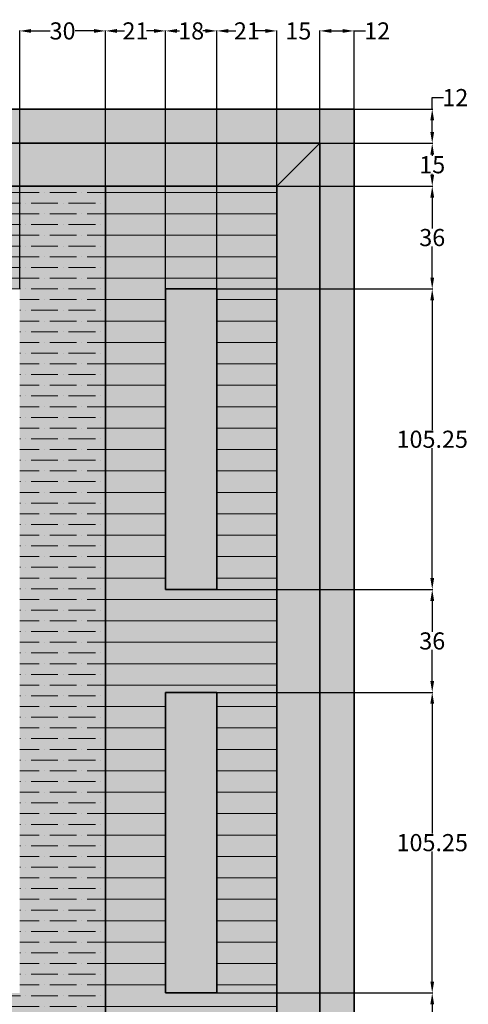
# Model space of a CAD drawing. Units: inches. Extents: x 184 to 649, y 215 to 818.
# Tile 9 of 9: x 492 to 649, y 473 to 818. Entities that reach past the tile are written whole.
import ezdxf

# ---------------------------------------------------------------- set-up
doc = ezdxf.new("R2010")
doc.units = ezdxf.units.IN
doc.header["$MEASUREMENT"] = 0
for name, color, linetype, lineweight in [('A-ANNO-DIMS', 2, 'Continuous', 18), ('A-ELEV', 7, 'Continuous', 35), ('A-ELEV-FILL', 9, 'Continuous', 13), ('A-ELEV-PATT', 8, 'Continuous', 13)]:
    doc.layers.add(name, color=color, linetype=linetype, lineweight=lineweight)
doc.styles.get("Standard").update_dxf_attribs({"font": 'arial.ttf'})
doc.dimstyles.get("Standard").update_dxf_attribs({"dimtxt": 6, "dimasz": 4, "dimexe": 0.18, "dimexo": 0.0625, "dimgap": 0.09, "dimtad": 0, "dimtih": 1, "dimtoh": 1, "dimdec": 0, "dimzin": 0, "dimdsep": 46, "dimlunit": 3, "dimtxsty": 'Standard', "dimcen": 0.09, "dimadec": 0, "dimazin": 0, "dimtfac": 1, "dimtdec": 0, "dimtofl": 0, "dimtmove": 0, "dimatfit": 3, "dimfxl": 1, "dimtolj": 1, "dimtzin": 0, "dimarcsym": 0})

# ---------------------------------------------------------------- blocks, each defined once
blk = doc.blocks.new('*D23')
at = {"layer": 'A-ANNO-DIMS', "color": 0, "lineweight": -2, "transparency": 16777216}
for p, q in [((472.97, 814.08), (468.97, 814.08)), ((476.97, 723.79), (476.97, 814.26)), ((491.97, 723.79), (491.97, 814.26)), ((495.97, 814.08), (499.97, 814.08))]:
    blk.add_line(p, q, dxfattribs=at)
at = {"layer": 'A-ANNO-DIMS', "color": 0, "transparency": 16777216}
for points in [[(472.97, 814.74), (472.97, 813.41), (476.97, 814.08)], [(495.97, 814.74), (495.97, 813.41), (491.97, 814.08)]]:
    blk.add_solid(points, dxfattribs=at)
at = {"layer": 'Defpoints', "color": 0, "transparency": 16777216}
for p in [(491.97, 814.08), (476.97, 723.73), (491.97, 723.73)]:
    blk.add_point(p, dxfattribs=at)
at = {"layer": 'A-ANNO-DIMS', "color": 0, "transparency": 16777216, "insert": (484.47, 814.08), "char_height": 6, "attachment_point": 5}
blk.add_mtext('\\A1;15', dxfattribs=at)
blk = doc.blocks.new('*D24')
at = {"layer": 'A-ANNO-DIMS', "color": 0, "lineweight": -2, "transparency": 16777216}
for p, q in [((491.97, 723.79), (491.97, 814.26)), ((495.97, 814.08), (502.6, 814.08)), ((517.97, 814.08), (511.35, 814.08)), ((521.97, 759.79), (521.97, 814.26))]:
    blk.add_line(p, q, dxfattribs=at)
at = {"layer": 'A-ANNO-DIMS', "color": 0, "transparency": 16777216}
for points in [[(495.97, 814.74), (495.97, 813.41), (491.97, 814.08)], [(517.97, 814.74), (517.97, 813.41), (521.97, 814.08)]]:
    blk.add_solid(points, dxfattribs=at)
at = {"layer": 'Defpoints', "color": 0, "transparency": 16777216}
for p in [(521.97, 814.08), (521.97, 759.73), (491.97, 723.73)]:
    blk.add_point(p, dxfattribs=at)
at = {"layer": 'A-ANNO-DIMS', "color": 0, "transparency": 16777216, "insert": (506.97, 814.08), "char_height": 6, "attachment_point": 5}
blk.add_mtext('\\A1;30', dxfattribs=at)
blk = doc.blocks.new('*D25')
at = {"layer": 'A-ANNO-DIMS', "color": 0, "lineweight": -2, "transparency": 16777216}
for p, q in [((521.97, 759.79), (521.97, 814.26)), ((525.97, 814.08), (528.61, 814.08)), ((538.97, 814.08), (536.33, 814.08)), ((542.97, 723.79), (542.97, 814.26))]:
    blk.add_line(p, q, dxfattribs=at)
at = {"layer": 'A-ANNO-DIMS', "color": 0, "transparency": 16777216}
for points in [[(525.97, 814.74), (525.97, 813.41), (521.97, 814.08)], [(538.97, 814.74), (538.97, 813.41), (542.97, 814.08)]]:
    blk.add_solid(points, dxfattribs=at)
at = {"layer": 'Defpoints', "color": 0, "transparency": 16777216}
for p in [(542.97, 814.08), (521.97, 759.73), (542.97, 723.73)]:
    blk.add_point(p, dxfattribs=at)
at = {"layer": 'A-ANNO-DIMS', "color": 0, "transparency": 16777216, "insert": (532.47, 814.08), "char_height": 6, "attachment_point": 5}
blk.add_mtext('\\A1;21', dxfattribs=at)
blk = doc.blocks.new('*D26')
at = {"layer": 'A-ANNO-DIMS', "color": 0, "lineweight": -2, "transparency": 16777216}
for p, q in [((542.97, 723.79), (542.97, 814.26)), ((546.97, 814.08), (547.86, 814.08)), ((556.97, 814.08), (556.08, 814.08)), ((560.97, 723.79), (560.97, 814.26))]:
    blk.add_line(p, q, dxfattribs=at)
at = {"layer": 'A-ANNO-DIMS', "color": 0, "transparency": 16777216}
for points in [[(546.97, 814.74), (546.97, 813.41), (542.97, 814.08)], [(556.97, 814.74), (556.97, 813.41), (560.97, 814.08)]]:
    blk.add_solid(points, dxfattribs=at)
at = {"layer": 'Defpoints', "color": 0, "transparency": 16777216}
for p in [(560.97, 814.08), (542.97, 723.73), (560.97, 723.73)]:
    blk.add_point(p, dxfattribs=at)
at = {"layer": 'A-ANNO-DIMS', "color": 0, "transparency": 16777216, "insert": (551.97, 814.08), "char_height": 6, "attachment_point": 5}
blk.add_mtext('\\A1;18', dxfattribs=at)
blk = doc.blocks.new('*D27')
at = {"layer": 'A-ANNO-DIMS', "color": 0, "lineweight": -2, "transparency": 16777216}
for p, q in [((560.97, 723.79), (560.97, 814.26)), ((564.97, 814.08), (567.61, 814.08)), ((577.97, 814.08), (575.33, 814.08)), ((581.97, 759.79), (581.97, 814.26))]:
    blk.add_line(p, q, dxfattribs=at)
at = {"layer": 'A-ANNO-DIMS', "color": 0, "transparency": 16777216}
for points in [[(564.97, 814.74), (564.97, 813.41), (560.97, 814.08)], [(577.97, 814.74), (577.97, 813.41), (581.97, 814.08)]]:
    blk.add_solid(points, dxfattribs=at)
at = {"layer": 'Defpoints', "color": 0, "transparency": 16777216}
for p in [(581.97, 814.08), (581.97, 759.73), (560.97, 723.73)]:
    blk.add_point(p, dxfattribs=at)
at = {"layer": 'A-ANNO-DIMS', "color": 0, "transparency": 16777216, "insert": (571.47, 814.08), "char_height": 6, "attachment_point": 5}
blk.add_mtext('\\A1;21', dxfattribs=at)
blk = doc.blocks.new('*D28')
at = {"layer": 'A-ANNO-DIMS', "color": 0, "lineweight": -2, "transparency": 16777216}
for p, q in [((577.97, 814.08), (573.97, 814.08)), ((581.97, 759.79), (581.97, 814.26)), ((596.97, 774.79), (596.97, 814.26)), ((600.97, 814.08), (604.97, 814.08))]:
    blk.add_line(p, q, dxfattribs=at)
at = {"layer": 'A-ANNO-DIMS', "color": 0, "transparency": 16777216}
for points in [[(577.97, 814.74), (577.97, 813.41), (581.97, 814.08)], [(600.97, 814.74), (600.97, 813.41), (596.97, 814.08)]]:
    blk.add_solid(points, dxfattribs=at)
at = {"layer": 'Defpoints', "color": 0, "transparency": 16777216}
for p in [(596.97, 814.08), (596.97, 774.73), (581.97, 759.73)]:
    blk.add_point(p, dxfattribs=at)
at = {"layer": 'A-ANNO-DIMS', "color": 0, "transparency": 16777216, "insert": (589.47, 814.08), "char_height": 6, "attachment_point": 5}
blk.add_mtext('\\A1;15', dxfattribs=at)
blk = doc.blocks.new('*D29')
at = {"layer": 'A-ANNO-DIMS', "color": 0, "lineweight": -2, "transparency": 16777216}
for p, q in [((596.97, 774.79), (596.97, 814.26)), ((600.97, 814.08), (604.97, 814.08)), ((608.97, 786.79), (608.97, 814.26)), ((608.97, 814.08), (612.97, 814.08))]:
    blk.add_line(p, q, dxfattribs=at)
at = {"layer": 'A-ANNO-DIMS', "color": 0, "transparency": 16777216}
for points in [[(600.97, 814.74), (600.97, 813.41), (596.97, 814.08)], [(604.97, 814.74), (604.97, 813.41), (608.97, 814.08)]]:
    blk.add_solid(points, dxfattribs=at)
at = {"layer": 'Defpoints', "color": 0, "transparency": 16777216}
for p in [(608.97, 814.08), (608.97, 786.73), (596.97, 774.73)]:
    blk.add_point(p, dxfattribs=at)
at = {"layer": 'A-ANNO-DIMS', "color": 0, "transparency": 16777216, "insert": (617.05, 814.08), "char_height": 6, "attachment_point": 5}
blk.add_mtext('\\A1;12', dxfattribs=at)
blk = doc.blocks.new('*D47')
at = {"layer": 'A-ANNO-DIMS', "color": 0, "lineweight": -2, "transparency": 16777216}
for p, q in [((561.04, 477.22), (636.5, 477.22)), ((636.32, 473.22), (636.32, 460.75)), ((636.32, 441.96), (636.32, 454.44)), ((582.04, 437.96), (636.5, 437.96))]:
    blk.add_line(p, q, dxfattribs=at)
at = {"layer": 'A-ANNO-DIMS', "color": 0, "transparency": 16777216}
for points in [[(635.66, 473.22), (636.99, 473.22), (636.32, 477.22)], [(635.66, 441.96), (636.99, 441.96), (636.32, 437.96)]]:
    blk.add_solid(points, dxfattribs=at)
at = {"layer": 'Defpoints', "color": 0, "transparency": 16777216}
for p in [(560.97, 477.22), (636.32, 477.22), (581.97, 437.96)]:
    blk.add_point(p, dxfattribs=at)
at = {"layer": 'A-ANNO-DIMS', "color": 0, "transparency": 16777216, "insert": (636.32, 457.59), "char_height": 6, "attachment_point": 5}
blk.add_mtext('\\A1;39.26', dxfattribs=at)
blk = doc.blocks.new('*D48')
at = {"layer": 'A-ANNO-DIMS', "color": 0, "lineweight": -2, "transparency": 16777216}
for p, q in [((561.04, 582.47), (636.5, 582.47)), ((636.32, 578.47), (636.32, 533)), ((636.32, 481.22), (636.32, 526.7)), ((561.04, 477.22), (636.5, 477.22))]:
    blk.add_line(p, q, dxfattribs=at)
at = {"layer": 'A-ANNO-DIMS', "color": 0, "transparency": 16777216}
for points in [[(635.66, 578.47), (636.99, 578.47), (636.32, 582.47)], [(635.66, 481.22), (636.99, 481.22), (636.32, 477.22)]]:
    blk.add_solid(points, dxfattribs=at)
at = {"layer": 'Defpoints', "color": 0, "transparency": 16777216}
for p in [(560.97, 582.47), (636.32, 582.47), (560.97, 477.22)]:
    blk.add_point(p, dxfattribs=at)
at = {"layer": 'A-ANNO-DIMS', "color": 0, "transparency": 16777216, "insert": (636.32, 529.85), "char_height": 6, "attachment_point": 5}
blk.add_mtext('\\A1;105.25', dxfattribs=at)
blk = doc.blocks.new('*D49')
at = {"layer": 'A-ANNO-DIMS', "color": 0, "lineweight": -2, "transparency": 16777216}
for p, q in [((561.04, 618.47), (636.5, 618.47)), ((636.32, 614.47), (636.32, 603.63)), ((636.32, 586.47), (636.32, 597.32)), ((561.04, 582.47), (636.5, 582.47))]:
    blk.add_line(p, q, dxfattribs=at)
at = {"layer": 'A-ANNO-DIMS', "color": 0, "transparency": 16777216}
for points in [[(635.66, 614.47), (636.99, 614.47), (636.32, 618.47)], [(635.66, 586.47), (636.99, 586.47), (636.32, 582.47)]]:
    blk.add_solid(points, dxfattribs=at)
at = {"layer": 'Defpoints', "color": 0, "transparency": 16777216}
for p in [(560.97, 618.47), (636.32, 618.47), (560.97, 582.47)]:
    blk.add_point(p, dxfattribs=at)
at = {"layer": 'A-ANNO-DIMS', "color": 0, "transparency": 16777216, "insert": (636.32, 600.47), "char_height": 6, "attachment_point": 5}
blk.add_mtext('\\A1;36', dxfattribs=at)
blk = doc.blocks.new('*D50')
at = {"layer": 'A-ANNO-DIMS', "color": 0, "lineweight": -2, "transparency": 16777216}
for p, q in [((561.04, 723.73), (636.5, 723.73)), ((636.32, 719.73), (636.32, 674.25)), ((636.32, 622.47), (636.32, 667.95)), ((561.04, 618.47), (636.5, 618.47))]:
    blk.add_line(p, q, dxfattribs=at)
at = {"layer": 'A-ANNO-DIMS', "color": 0, "transparency": 16777216}
for points in [[(635.66, 719.73), (636.99, 719.73), (636.32, 723.73)], [(635.66, 622.47), (636.99, 622.47), (636.32, 618.47)]]:
    blk.add_solid(points, dxfattribs=at)
at = {"layer": 'Defpoints', "color": 0, "transparency": 16777216}
for p in [(560.97, 723.73), (636.32, 723.73), (560.97, 618.47)]:
    blk.add_point(p, dxfattribs=at)
at = {"layer": 'A-ANNO-DIMS', "color": 0, "transparency": 16777216, "insert": (636.32, 671.1), "char_height": 6, "attachment_point": 5}
blk.add_mtext('\\A1;105.25', dxfattribs=at)
blk = doc.blocks.new('*D51')
at = {"layer": 'A-ANNO-DIMS', "color": 0, "lineweight": -2, "transparency": 16777216}
for p, q in [((582.04, 759.73), (636.5, 759.73)), ((636.32, 755.73), (636.32, 744.88)), ((636.32, 727.73), (636.32, 738.57)), ((561.04, 723.73), (636.5, 723.73))]:
    blk.add_line(p, q, dxfattribs=at)
at = {"layer": 'A-ANNO-DIMS', "color": 0, "transparency": 16777216}
for points in [[(635.66, 755.73), (636.99, 755.73), (636.32, 759.73)], [(635.66, 727.73), (636.99, 727.73), (636.32, 723.73)]]:
    blk.add_solid(points, dxfattribs=at)
at = {"layer": 'Defpoints', "color": 0, "transparency": 16777216}
for p in [(581.97, 759.73), (636.32, 759.73), (560.97, 723.73)]:
    blk.add_point(p, dxfattribs=at)
at = {"layer": 'A-ANNO-DIMS', "color": 0, "transparency": 16777216, "insert": (636.32, 741.73), "char_height": 6, "attachment_point": 5}
blk.add_mtext('\\A1;36', dxfattribs=at)
blk = doc.blocks.new('*D52')
at = {"layer": 'A-ANNO-DIMS', "color": 0, "lineweight": -2, "transparency": 16777216}
for p, q in [((597.04, 774.73), (636.5, 774.73)), ((636.32, 770.73), (636.32, 770.38)), ((636.32, 763.73), (636.32, 764.07)), ((582.04, 759.73), (636.5, 759.73))]:
    blk.add_line(p, q, dxfattribs=at)
at = {"layer": 'A-ANNO-DIMS', "color": 0, "transparency": 16777216}
for points in [[(635.66, 770.73), (636.99, 770.73), (636.32, 774.73)], [(635.66, 763.73), (636.99, 763.73), (636.32, 759.73)]]:
    blk.add_solid(points, dxfattribs=at)
at = {"layer": 'Defpoints', "color": 0, "transparency": 16777216}
for p in [(596.97, 774.73), (636.32, 774.73), (581.97, 759.73)]:
    blk.add_point(p, dxfattribs=at)
at = {"layer": 'A-ANNO-DIMS', "color": 0, "transparency": 16777216, "insert": (636.32, 767.23), "char_height": 6, "attachment_point": 5}
blk.add_mtext('\\A1;15', dxfattribs=at)
blk = doc.blocks.new('*D53')
at = {"layer": 'A-ANNO-DIMS', "color": 0, "lineweight": -2, "transparency": 16777216}
for p, q in [((636.32, 786.73), (636.32, 790.73)), ((636.32, 790.73), (640.32, 790.73)), ((609.04, 786.73), (636.5, 786.73)), ((636.32, 778.73), (636.32, 782.73)), ((597.04, 774.73), (636.5, 774.73))]:
    blk.add_line(p, q, dxfattribs=at)
at = {"layer": 'A-ANNO-DIMS', "color": 0, "transparency": 16777216}
for points in [[(635.66, 782.73), (636.99, 782.73), (636.32, 786.73)], [(635.66, 778.73), (636.99, 778.73), (636.32, 774.73)]]:
    blk.add_solid(points, dxfattribs=at)
at = {"layer": 'Defpoints', "color": 0, "transparency": 16777216}
for p in [(608.97, 786.73), (636.32, 786.73), (596.97, 774.73)]:
    blk.add_point(p, dxfattribs=at)
at = {"layer": 'A-ANNO-DIMS', "color": 0, "transparency": 16777216, "insert": (644.4, 790.73), "char_height": 6, "attachment_point": 5}
blk.add_mtext('\\A1;12', dxfattribs=at)

msp = doc.modelspace()

# ---------------------------------------------------------------- hatches: boundary and pattern name
at = {"layer": 'A-ELEV-FILL'}
h = msp.add_hatch(color=256, dxfattribs=at)
h.dxf.hatch_style = 1
h.paths.add_polyline_path([(608.9726, 786.7265), (452.9726, 786.7265), (360.1071, 692.7265), (372.3627, 692.7265), (452.9726, 774.7265), (596.9726, 774.7265), (596.9726, 369.7265), (581.9726, 369.7265), (581.9726, 282.7265), (594.8393, 246.7265), (608.9726, 246.7265)])
h = msp.add_hatch(color=256, dxfattribs=at)
h.dxf.hatch_style = 1
h.paths.add_polyline_path([(596.9726, 774.7265), (452.9726, 774.7265), (372.3627, 692.7265), (386.4196, 692.7265), (452.9726, 759.7265), (581.9726, 759.7265)])
h = msp.add_hatch(color=256, dxfattribs=at)
h.dxf.hatch_style = 1
h.paths.add_polyline_path([(596.9726, 774.7265), (581.9726, 759.7265), (581.9726, 437.9607), (573.4578, 437.9607), (573.4578, 431.9607), (569.4578, 431.9607), (569.4578, 425.9607), (565.4578, 425.9607), (565.4578, 419.9607), (561.4578, 419.9607), (561.4578, 413.9607), (557.4578, 413.9607), (557.4578, 407.9607), (553.4578, 407.9607), (553.4578, 401.9607), (549.4578, 401.9607), (549.4578, 395.9607), (545.4578, 395.9607), (545.4578, 389.9607), (541.4578, 389.9607), (541.4578, 383.9607), (537.4578, 383.9607), (537.4578, 377.9607), (533.4578, 377.9607), (533.4578, 371.9607), (529.4578, 371.9607), (529.4578, 369.7265), (596.9726, 369.7265)])
h = msp.add_hatch(color=256, dxfattribs=at)
h.dxf.hatch_style = 1
h.paths.add_polyline_path([(380.9726, 453.5037), (422.2268, 453.5037), (422.2268, 474.7265), (260.9726, 474.7265), (260.9726, 369.7265), (291.9998, 369.7265), (291.9998, 453.5037), (339.9998, 453.5037), (339.9998, 369.7265), (380.9726, 369.7265)])
h.paths.add_polyline_path([(437.9726, 328.7265), (275.9726, 328.7265), (275.9726, 246.7265), (437.9726, 246.7265)])
h.paths.add_polyline_path([(581.9726, 759.7265), (521.9726, 759.7265), (521.9726, 441.2233), (581.9726, 441.2233)])
h.paths.add_polyline_path([(560.9726, 582.4749), (560.9726, 477.2233), (542.9726, 477.2233), (542.9726, 582.4749)], flags=16)
h.paths.add_polyline_path([(560.9726, 618.4749), (542.9726, 618.4749), (542.9726, 723.7265), (560.9726, 723.7265)], flags=16)
h = msp.add_hatch(color=256, dxfattribs=at)
h.dxf.hatch_style = 1
h.paths.add_polyline_path([(521.9726, 759.7265), (452.9726, 759.7265), (452.9726, 441.2233), (521.9726, 441.2233)])
h.paths.add_polyline_path([(491.9726, 477.2233), (476.9726, 477.2233), (476.9726, 723.7265), (491.9726, 723.7265)], flags=16)
h = msp.add_hatch(color=256, dxfattribs=at)
h.dxf.hatch_style = 1
h.paths.add_polyline_path([(560.9726, 723.7265), (542.9726, 723.7265), (542.9726, 618.4749), (560.9726, 618.4749)])
h.paths.add_polyline_path([(560.9726, 582.4749), (542.9726, 582.4749), (542.9726, 477.2233), (560.9726, 477.2233)])
at = {"layer": 'A-ELEV-PATT'}
h = msp.add_hatch(dxfattribs=at)
h.set_pattern_fill('ANSI36', color=256, scale=30, angle=135)
h.paths.add_polyline_path([(521.9726, 759.7265), (452.9726, 759.7265), (452.9726, 441.2233), (521.9726, 441.2233)])
h.paths.add_polyline_path([(476.9726, 723.7265), (491.9726, 723.7265), (491.9726, 477.2233), (476.9726, 477.2233)], flags=16)
h = msp.add_hatch(dxfattribs=at)
h.set_pattern_fill('ANSI31', color=256, scale=60, angle=135)
h.paths.add_polyline_path([(581.9726, 759.7265), (521.9726, 759.7265), (521.9726, 441.2233), (581.9726, 441.2233)])
h.paths.add_polyline_path([(560.9726, 723.7265), (560.9726, 618.4749), (542.9726, 618.4749), (542.9726, 723.7265)], flags=16)
h.paths.add_polyline_path([(560.9726, 582.4749), (560.9726, 477.2233), (542.9726, 477.2233), (542.9726, 582.4749)], flags=16)

# ---------------------------------------------------------------- linework, layer by layer
at = {"layer": 'A-ELEV'}
for p, q in [((608.9726, 786.7265), (248.9726, 786.7265)), ((608.9726, 246.7265), (608.9726, 786.7265)), ((596.9726, 774.7265), (452.9726, 774.7265)), ((596.9726, 774.7265), (581.9726, 759.7265)), ((596.9726, 369.7265), (596.9726, 774.7265)), ((581.9726, 759.7265), (452.9726, 759.7265)), ((521.9726, 441.2233), (521.9726, 759.7265)), ((581.9726, 437.9607), (581.9726, 759.7265)), ((542.9726, 723.7265), (560.9726, 723.7265)), ((542.9726, 618.4749), (542.9726, 723.7265)), ((560.9726, 618.4749), (560.9726, 723.7265)), ((542.9726, 618.4749), (560.9726, 618.4749)), ((542.9726, 477.2233), (542.9726, 582.4749)), ((542.9726, 582.4749), (560.9726, 582.4749)), ((560.9726, 477.2233), (560.9726, 582.4749)), ((542.9726, 477.2233), (560.9726, 477.2233))]:
    msp.add_line(p, q, dxfattribs=at)

# ---------------------------------------------------------------- dimensions: what is measured, and where the dimension line sits
at = {"layer": 'A-ANNO-DIMS'}
for base, p1, p2, picture, middle in [((491.9726, 814.0765), (476.9726, 723.7265), (491.9726, 723.7265), '*D23', (484.4726, 814.0765)), ((521.9726, 814.0765), (491.9726, 723.7265), (521.9726, 759.7265), '*D24', (506.9726, 814.0765)), ((542.9726, 814.0765), (521.9726, 759.7265), (542.9726, 723.7265), '*D25', (532.4726, 814.0765)), ((560.9726, 814.0765), (542.9726, 723.7265), (560.9726, 723.7265), '*D26', (551.9726, 814.0765)), ((581.9726, 814.0765), (560.9726, 723.7265), (581.9726, 759.7265), '*D27', (571.4726, 814.0765)), ((596.9726, 814.0765), (581.9726, 759.7265), (596.9726, 774.7265), '*D28', (589.4726, 814.0765)), ((608.9726, 814.0765), (596.9726, 774.7265), (608.9726, 786.7265), '*D29', (617.0469, 814.0765))]:
    dim = msp.add_linear_dim(base=base, p1=p1, p2=p2, dimstyle='Standard', override={"dimdec": 0, "dimlfac": 1, "dimrnd": 0, "dimzin": 0, "dimdsep": 46, "dimlunit": 2}, dxfattribs=at)
    dim.commit()
    dim.dimension.update_dxf_attribs({"geometry": picture, "text_midpoint": middle})
for base, p1, p2, override, picture, middle in [((636.3226, 786.7265), (596.9726, 774.7265), (608.9726, 786.7265), {"dimdec": 0, "dimlfac": 1, "dimrnd": 0, "dimzin": 0, "dimdsep": 46, "dimlunit": 2}, '*D53', (644.3969, 790.7265)), ((636.3226, 774.7265), (581.9726, 759.7265), (596.9726, 774.7265), {"dimdec": 0, "dimlfac": 1, "dimrnd": 0, "dimzin": 0, "dimdsep": 46, "dimlunit": 2}, '*D52', (636.3226, 767.2265)), ((636.3226, 759.7265), (560.9726, 723.7265), (581.9726, 759.7265), {"dimdec": 0, "dimlfac": 1, "dimrnd": 0, "dimzin": 0, "dimdsep": 46, "dimlunit": 2}, '*D51', (636.3226, 741.7265)), ((636.3226, 723.7265), (560.9726, 618.4749), (560.9726, 723.7265), {"dimdec": 2, "dimlfac": 1, "dimrnd": 0, "dimzin": 0, "dimdsep": 46, "dimlunit": 2}, '*D50', (636.3226, 671.1007)), ((636.3226, 618.4749), (560.9726, 582.4749), (560.9726, 618.4749), {"dimdec": 0, "dimlfac": 1, "dimrnd": 0, "dimzin": 0, "dimdsep": 46, "dimlunit": 2}, '*D49', (636.3226, 600.4749)), ((636.3226, 582.4749), (560.9726, 477.2233), (560.9726, 582.4749), {"dimdec": 2, "dimlfac": 1, "dimrnd": 0, "dimzin": 0, "dimdsep": 46, "dimlunit": 2}, '*D48', (636.3226, 529.8491)), ((636.3226, 477.2233), (581.9726, 437.9607), (560.9726, 477.2233), {"dimdec": 2, "dimlfac": 1, "dimrnd": 0, "dimzin": 0, "dimdsep": 46, "dimlunit": 2}, '*D47', (636.3226, 457.592))]:
    dim = msp.add_linear_dim(base=base, p1=p1, p2=p2, angle=90, dimstyle='Standard', override=override, dxfattribs=at)
    dim.commit()
    dim.dimension.update_dxf_attribs({"geometry": picture, "text_midpoint": middle})

doc.saveas('drawing.dxf')
